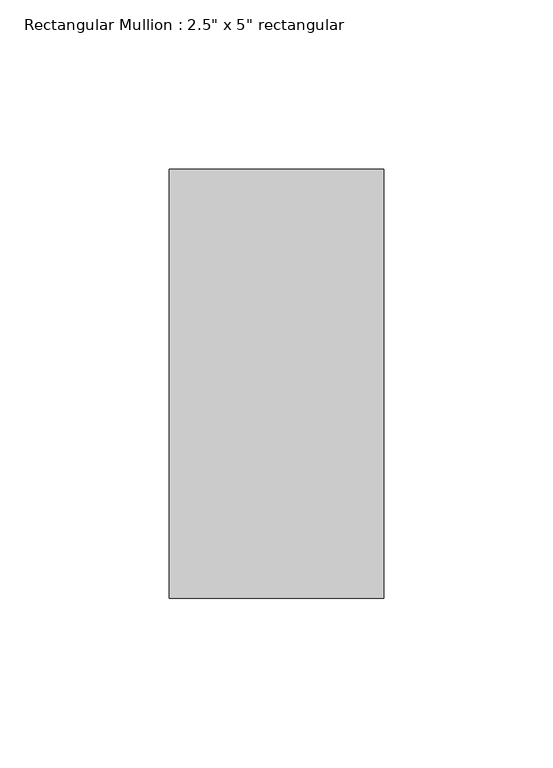
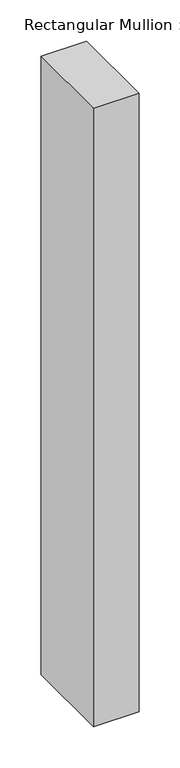
"""IFC4 building model written with IfcOpenShell, lengths in millimetres: member geometry."""

from ifc_helpers import new_model, si_unit, frame, origin, place, context, project, spatial, polyline, outline, extrude, source, transform, mapped, element, save


def member_410c6227(model_context):
    return source(origin(), model_context, "Body", "SweptSolid", [
        extrude(outline(polyline([(31.75, 63.5), (31.75, -63.5), (-31.75, -63.5), (-31.75, 63.5), (31.75, 63.5)])), frame((0.0, 0.0, -914.4), z_axis=(0.0, 0.0, 1.0), x_axis=(1.0, 0.0, 0.0)), (0.0, 0.0, 1.0), 914.4),
    ])


if __name__ == "__main__":
    model = new_model("IFC4")
    model_context = context("Model", 3, world=origin())
    ifc_project = project(units=[si_unit("LENGTHUNIT", "METRE", prefix="MILLI")], contexts=[model_context])
    site = spatial("IfcSite", under=ifc_project)
    building = spatial("IfcBuilding", under=site)
    placement = place(None, origin())
    member_shape = member_410c6227(model_context)
    element("IfcMember", 1, ObjectType="Rectangular Mullion : 2.5\" x 5\" rectangular", at=placement, inside=building, context=model_context, shape_type="MappedRepresentation", body=[
        mapped(member_shape, transform((0.0, 0.0, 0.0), x_axis=(1.0, 0.0, 0.0), y_axis=(0.0, 1.0, 0.0), z_axis=(0.0, 0.0, 1.0))),
    ])
    save(model, "model.ifc")

# Revit data of these elements
# Type "Rectangular Mullion : 2.5\" x 5\" rectangular"
#   built-in parameter 1007304 = 0.416667 (stored number, unit not read)
#   built-in parameter 1007301 = 0.104167 (stored number, unit not read)
#   built-in parameter 1007300 = 0.104167 (stored number, unit not read)
# Element 1 (IfcMember, "Rectangular Mullion : 2.5\" x 5\" rectangular")
#   Materials on its faces: "WINDOW FRAMING"
# Materials
#   "WINDOW FRAMING": class "Generic", colour RGB 120 120 120, transparency 0, Cost = 0
